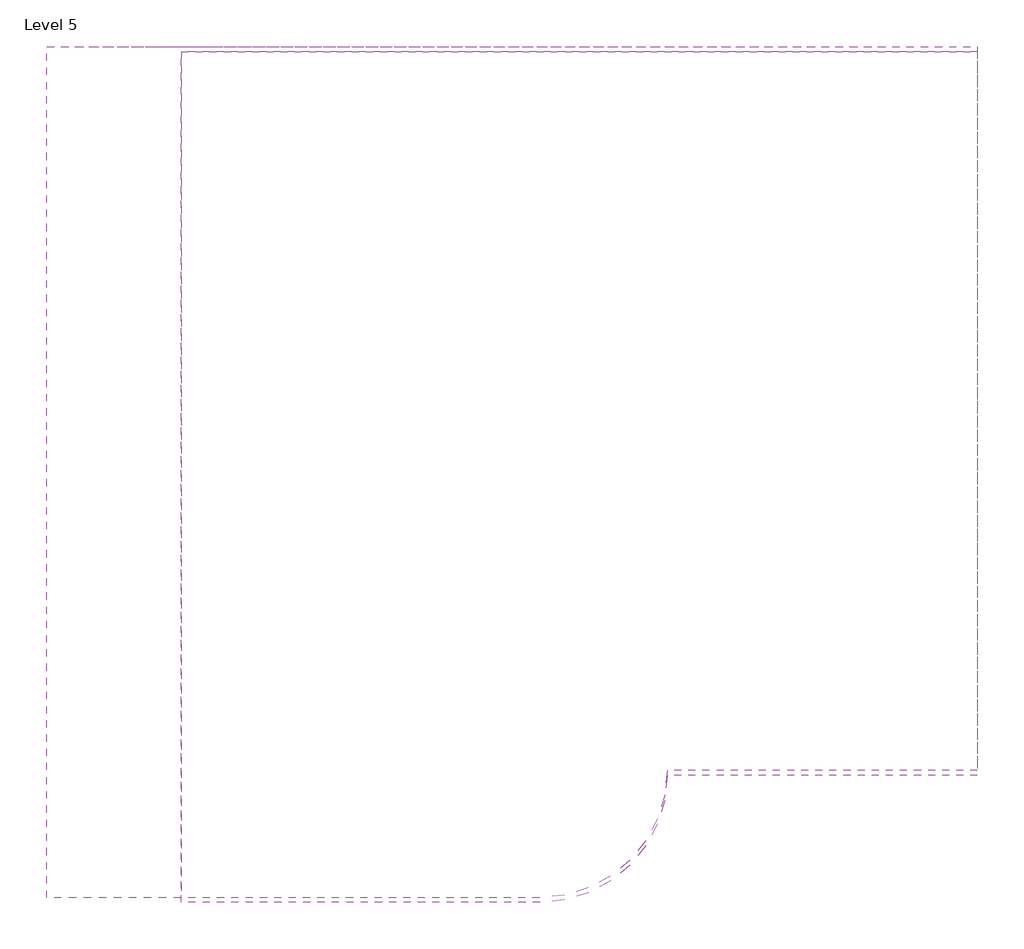
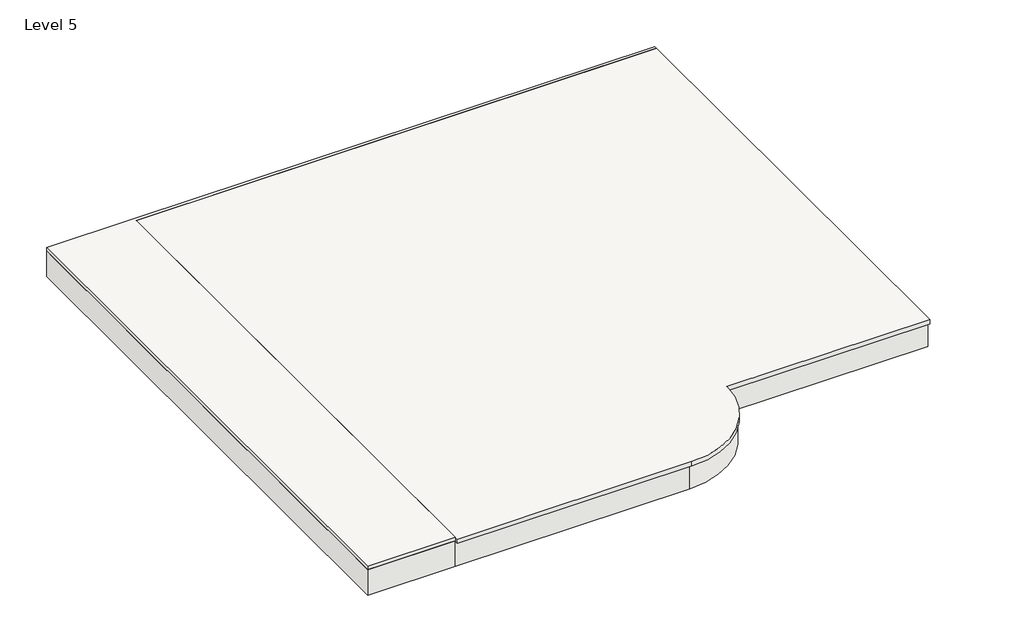
# One storey: 3 slabs.
"""IFC4 building model written with IfcOpenShell, lengths in millimetres."""

from ifc_helpers import new_model, si_unit, point, frame, frame_2d, origin, place, context, project, spatial, polyline, circle_curve, trimmed, segment, composite_curve, outline, extrude, element, save

model = new_model("IFC4")

# Units and contexts
model_context = context("Model", 3, world=origin())
ifc_project = project(units=[si_unit("LENGTHUNIT", "METRE", prefix="MILLI")], contexts=[model_context])

# Site, building, storey
site = spatial("IfcSite", under=ifc_project)
building = spatial("IfcBuilding", under=site)
storey = spatial("IfcBuildingStorey", under=building, Name="Level 5", Elevation=12192.0)

# Slabs
placement = place(None, origin())
element("IfcSlab", 1, ObjectType="Generic - 4\"", at=placement, inside=storey, context=model_context, shape_type="SweptSolid", body=[
    extrude(outline(polyline([(-17203.0104559, 11493.328737), (-5468.2104559, 11493.328737), (-5468.2104559, 11417.128737), (-17203.0104559, 11417.128737), (-17203.0104559, -1054.271263), (-19184.2104559, -1054.271263), (-19184.2104559, 11493.328737), (-17203.0104559, 11493.328737)])), frame((0.0, 0.0, 14757.4), z_axis=(0.0, 0.0, 1.0), x_axis=(1.0, 0.0, 0.0)), (0.0, 0.0, 1.0), 101.6),
])
element("IfcSlab", 2, ObjectType="LW Concrete on Metal Deck", at=placement, inside=storey, context=model_context, shape_type="SweptSolid", body=[
    extrude(outline(composite_curve([segment(polyline([(-5468.2104559, 11417.128737), (-5468.2104559, 749.128737), (-10040.2104559, 749.128737)]), True, "CONTINUOUS"), segment(trimmed(circle_curve(frame_2d((-11913.4604559, 749.128737)), 1873.25), [point((-10040.2104559, 749.128737))], [point((-11913.4604559, -1124.121263))], False, "CARTESIAN"), True, "CONTINUOUS"), segment(polyline([(-11913.4604559, -1124.121263), (-17203.0104559, -1124.121263), (-17203.0104559, 11417.128737), (-5468.2104559, 11417.128737)]), True, "CONTINUOUS")], self_intersect=False)), frame((0.0, 0.0, 14754.225), z_axis=(0.0, 0.0, 1.0), x_axis=(1.0, 0.0, 0.0)), (0.0, 0.0, 1.0), 104.775),
])
element("IfcSlab", 3, ObjectType="wall design 2", at=placement, inside=storey, context=model_context, shape_type="SweptSolid", body=[
    extrude(outline(composite_curve([segment(polyline([(-5468.2104559, 11493.328737), (-5468.2104559, 825.328737), (-10040.2104559, 825.328737)]), True, "CONTINUOUS"), segment(trimmed(circle_curve(frame_2d((-11919.8104559, 825.328737)), 1879.6), [point((-10040.2104559, 825.328737))], [point((-11919.8104559, -1054.271263))], False, "CARTESIAN"), True, "CONTINUOUS"), segment(polyline([(-11919.8104559, -1054.271263), (-17203.0104559, -1054.271263), (-19184.2104559, -1054.271263), (-19184.2104559, 11493.328737), (-5468.2104559, 11493.328737)]), True, "CONTINUOUS")], self_intersect=False)), frame((0.0, 0.0, 14173.2), z_axis=(0.0, 0.0, 1.0), x_axis=(1.0, 0.0, 0.0)), (0.0, 0.0, 1.0), 609.6),
])

save(model, "model.ifc")

# Revit data of these elements
# Type "Generic - 4\""
#   Assembly Code = "B1010"
#   Function = 0
#   Layers, outside or top first: 0' - 4" "Parking Stripe" (function 1)
# Type "LW Concrete on Metal Deck"
#   Assembly Code = "B1010"
#   Function = 0
#   Layers, outside or top first: 0' - 4" "Concrete, Lightweight" (function 1); 0' - 0 1/8" "Default Mass Opening" (function 1)
# Type "wall design 2"
#   Assembly Code = "B1010"
#   Function = 0
#   Layers, outside or top first: 2' - 0" "Damp-proofing" (function 1)
# Element 1 (IfcSlab, "Generic - 4\"")
#   Height Offset From Level = 8' - 9"
#   Phase Created = New Construction
#   Materials on its faces: "Parking Stripe"
# Element 2 (IfcSlab, "LW Concrete on Metal Deck")
#   Height Offset From Level = 8' - 9"
#   Phase Created = New Construction
#   Materials on its faces: "Default Mass Opening", "Concrete, Lightweight"
# Element 3 (IfcSlab, "wall design 2")
#   Height Offset From Level = 8' - 6"
#   Phase Created = New Construction
#   Materials on its faces: "Damp-proofing"
# Materials
#   "Parking Stripe": class "Paint", colour RGB 250 250 91, transparency 0, Cost = 0
#   "Concrete, Lightweight": class "Concrete", colour RGB 142 141 140, transparency 0, Description = "Lightweight concrete", Cost = 0
#   "Default Mass Opening": class "Generic", colour RGB 255 255 255, transparency 1, Cost = 0
#   "Damp-proofing": class "Generic", colour RGB 127 127 127, transparency 0, Description = "Damp-proofing", Cost = 0
